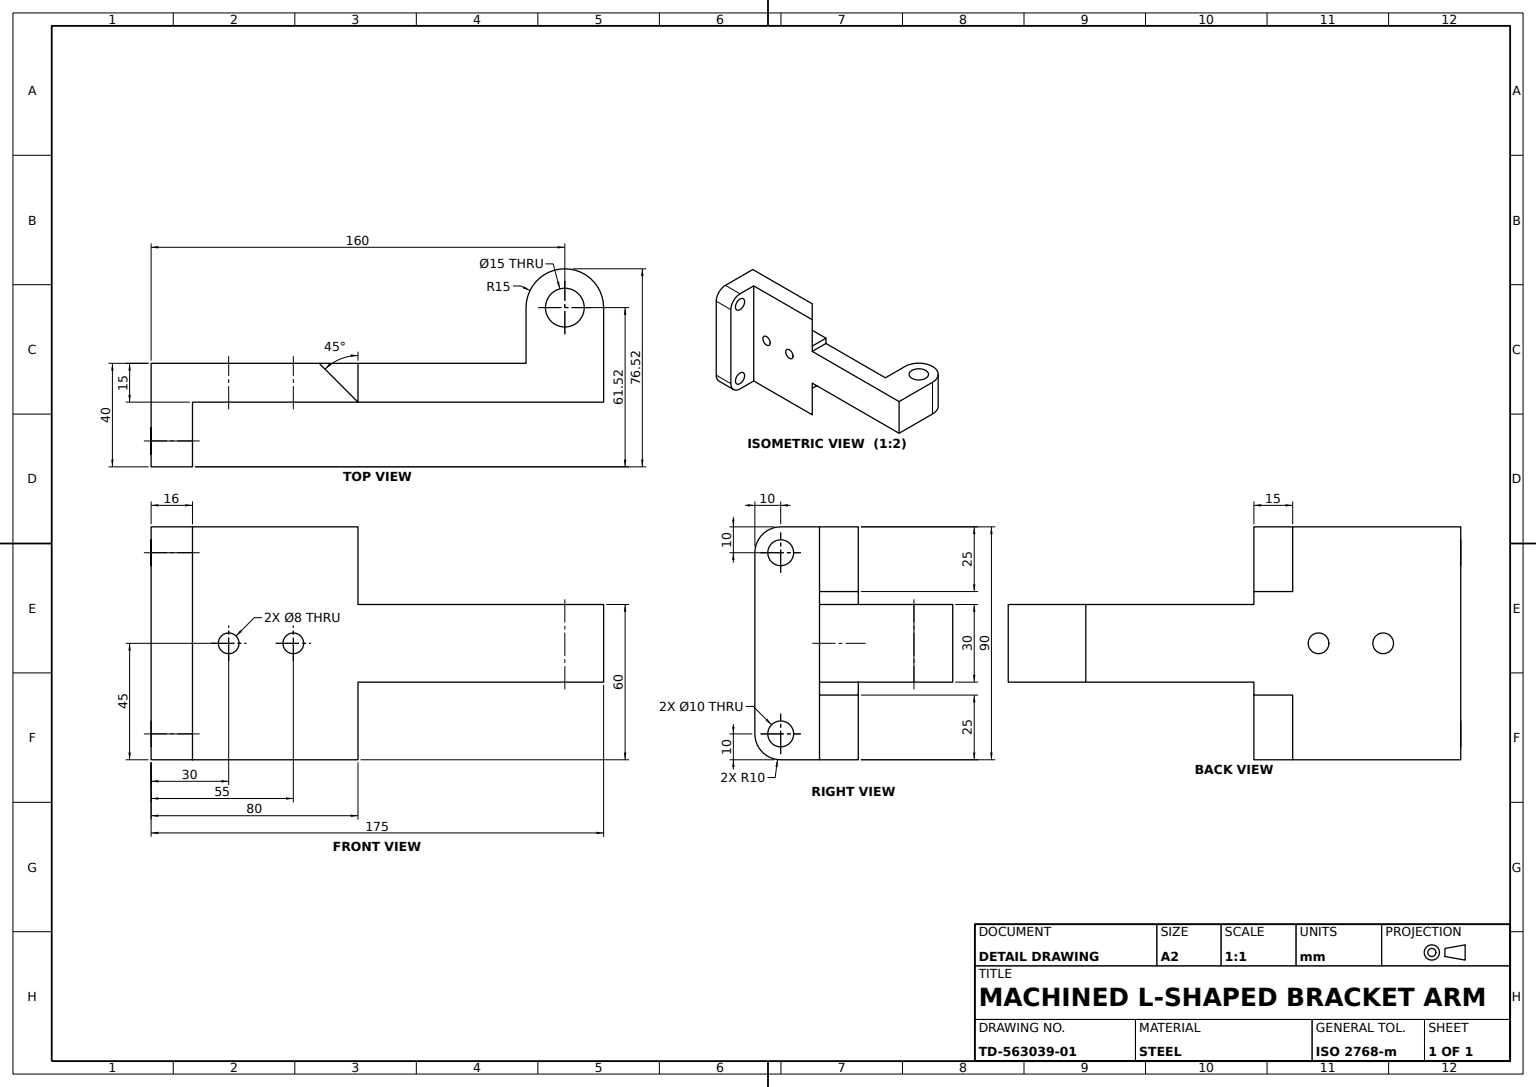
SolidWorks part; units mm, degrees
material "Plain Carbon Steel"
ref_plane "Front Plane" through (0, 0, 0) normal (0, 0, 1) x (1, 0, 0)
ref_plane "Top Plane" through (0, 0, 0) normal (0, 1, 0) x (1, 0, 0)
ref_plane "Right Plane" through (0, 0, 0) normal (1, 0, 0) x (0, 0, -1)
sketch "Bracket Profile Sketch" plane through (0, 0, 0) normal (0, 1, 0) x (1, 0, 0)
  line L0 (-24, -7.5) -> (-24, -32.5)
  line L1 (-24, 7.5) -> (40, 7.5)
  line L3 (-24, -7.5) -> (40, -7.5)
  line L4 (40, 7.5) -> (40, -7.5)
  line L7 (-40, 7.5) -> (-24, 7.5)
  line L8 (-40, 7.5) -> (-40, -32.5)
  line L9 (-40, -32.5) -> (-24, -32.5)
  point P0 (0, 0)
  dimension "D1" = 16
  dimension "D2" = 40
  dimension "D3" = 15
  dimension "D4" = 40
  dimension "D5" = 80
  dimension "D6" = 32.5
extrude "Bracket Body" add sketch "Bracket Profile Sketch" along normal blind 90
sketch "Angled Cut Sketch" plane through (0, 90, 0) normal (0, 1, 0) x (1, 0, 0)
  line L0 (25, 7.5) -> (40, -7.5)
  line L6 (40, -7.5) -> (40, 7.5)
  line L7 (40, 7.5) -> (-40, 7.5)
  line L8 (-40, 7.5) -> (-40, -32.5)
  line L9 (-40, -32.5) -> (-24, -32.5)
  line L10 (-24, -32.5) -> (-24, -7.5)
  line L11 (-24, -7.5) -> (40, -7.5)
  line L12 (40, -7.5) -> (40, 7.5)
  line L13 (40, 7.5) -> (-40, 7.5)
  line L14 (-40, 7.5) -> (-40, -32.5)
  line L15 (-40, -32.5) -> (-24, -32.5)
  line L16 (-24, -32.5) -> (-24, -7.5)
  line L17 (-24, -7.5) -> (40, -7.5)
  line M8 (40, -7.5) -> (40, 7.5)
  line M9 (40, 7.5) -> (-40, 7.5)
  dimension "D2" = 45
  dimension "D1" = 0
extrude "Angled Cut" cut sketch "Angled Cut Sketch" against normal blind 25 contours L0 M9 M8
ref_plane "Bracket Mid Plane" through (0, 45, 0) normal (0, 1, 0) x (1, 0, 0)
mirror "Angled Cut Mirror" about plane through (0, 45, 0) normal (0, 1, 0) of "Angled Cut"
sketch "Arm Boss Sketch" plane through (0, 45, 0) normal (0, 1, 0) x (1, 0, 0)
  line L0 (40, 7.5) -> (25, 7.5) construction
  line L1 (40, -7.5) -> (135, -7.5)
  line L2 (40, -7.5) -> (40, 7.5)
  line L3 (40, 7.5) -> (105, 7.5)
  line L7 (105, 29.0249) -> (105, 7.5)
  line L10 (135, 29.0249) -> (135, -7.5)
  arc A2 (135, 29.0249) -> (105, 29.0249) centre (120, 29.0249) ccw
  circle A3 centre (120, 29.0249) radius 7.5
  dimension "D2" = 30
  dimension "D3" = 15
  dimension "D4" = 29.0249
  dimension "D1" = 120
extrude "Arm Boss" add sketch "Arm Boss Sketch" along normal mid plane 30
fillet "Corner Fillets R10" radius 10 2 edges at (-32, 0, 32.5) (-32, 90, 32.5)
sketch "Corner Holes Sketch" plane through (-40, 0, 0) normal (-1, 0, 0) x (0, 0, 1)
  circle A0 centre (22.5, 80) radius 5
  circle A1 centre (22.5, 10) radius 5
  arc A2 (32.5, 80) -> (22.5, 90) centre (22.5, 80) ccw construction
  arc A3 (22.5, 0) -> (32.5, 10) centre (22.5, 10) ccw construction
  dimension "D1" = 10
extrude "Corner Holes Ø10" cut sketch "Corner Holes Sketch" against normal through all both and the other way through all
sketch "Face Holes Sketch" plane through (0, 0, -7.5) normal (0, 0, -1) x (-1, 0, 0)
  line L0 (40, 90) -> (40, 0) construction
  line L1 (-25, 0) -> (40, 0) construction
  circle A0 centre (10, 45) radius 4
  circle A1 centre (-15, 45) radius 4
  dimension "D1" = 8
  dimension "D2" = 30
  dimension "D3" = 25
  dimension "D4" = 45
extrude "Face Holes 2xØ8" cut sketch "Face Holes Sketch" against normal through all both and the other way through all
